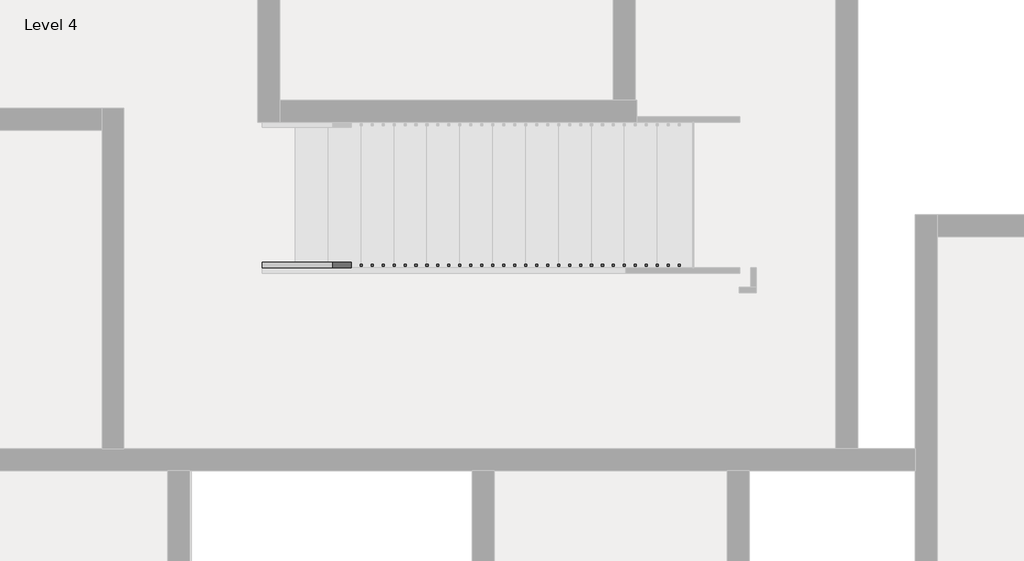
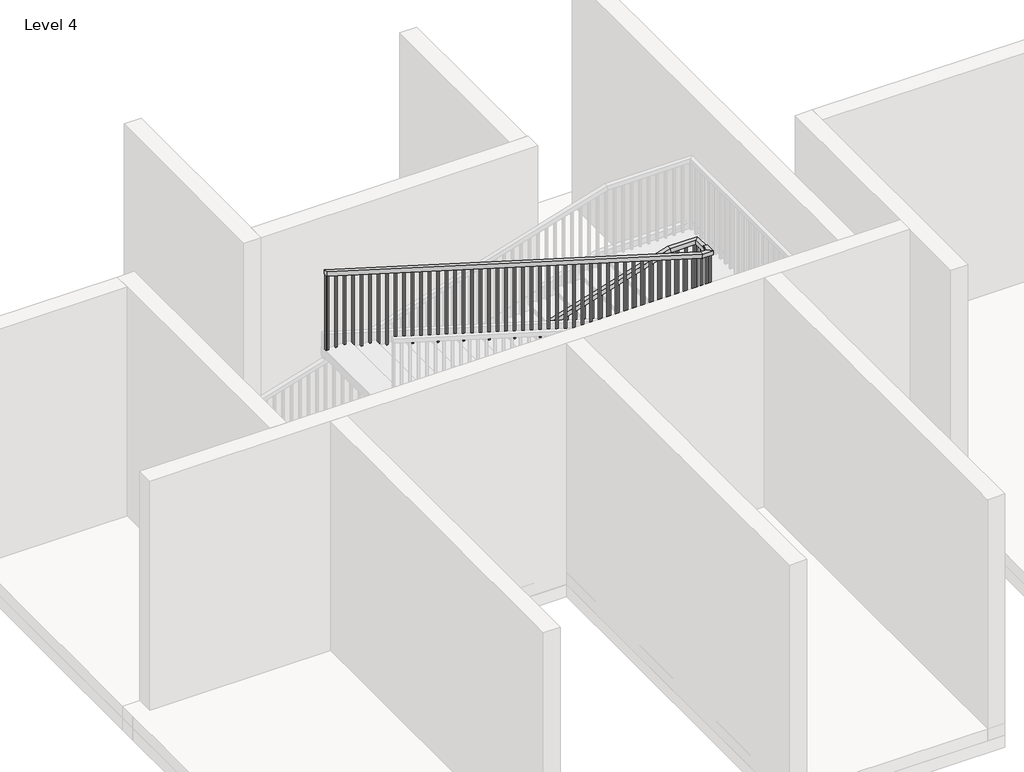
# One storey, part 11 of 14: 1 railing.
"""IFC4 building model written with IfcOpenShell, lengths in millimetres."""

from ifc_helpers import new_model, si_unit, frame, origin, place, context, project, spatial, polyline, outline, extrude, faceted_brep, element, save

model = new_model("IFC4")

# Units and contexts
model_context = context("Model", 3, world=origin())
ifc_project = project(units=[si_unit("LENGTHUNIT", "METRE", prefix="MILLI")], contexts=[model_context])

# Site, building, storey
site = spatial("IfcSite", under=ifc_project)
building = spatial("IfcBuilding", under=site)
storey = spatial("IfcBuildingStorey", under=building, Name="Level 4", Elevation=9144.0)

# Railing
placement = place(None, origin())
element("IfcRailing", 1, ObjectType="Handrail - Rectangular", at=placement, inside=storey, context=model_context, shape_type="SolidModel", body=[
    faceted_brep([(-5254.0891351, 11205.0082924, 10149.84), (-5254.0891351, 11205.0082924, 10096.8032429), (-5254.0891351, 11154.2082924, 10096.8032429), (-5254.0891351, 11154.2082924, 10149.84), (-986.8891351, 11205.0082924, 11430.0), (-979.4332782, 11205.0082924, 11379.2), (-979.4332782, 11154.2082924, 11379.2), (-986.8891351, 11154.2082924, 11430.0), (-631.2891351, 11205.0082924, 11430.0), (-631.2891351, 11205.0082924, 11379.2), (-682.0891351, 11154.2082924, 11379.2), (-682.0891351, 11154.2082924, 11430.0), (-631.2891351, 11001.8082924, 11430.0), (-631.2891351, 10951.0082924, 11379.2), (-682.0891351, 10951.0082924, 11379.2), (-682.0891351, 11001.8082924, 11430.0), (-631.2891351, 11001.8082924, 11452.86), (-631.2891351, 10951.0082924, 11402.06), (-682.0891351, 10951.0082924, 11402.06), (-682.0891351, 11001.8082924, 11452.86), (-631.2891351, 10874.8082924, 11452.86), (-631.2891351, 10874.8082924, 11402.06), (-682.0891351, 10925.6082924, 11402.06), (-682.0891351, 10925.6082924, 11452.86), (-758.2891351, 10874.8082924, 11452.86), (-765.744992, 10874.8082924, 11402.06), (-765.744992, 10925.6082924, 11402.06), (-758.2891351, 10925.6082924, 11452.86), (-5254.0891351, 10874.8082924, 12801.6), (-5254.0891351, 10925.6082924, 12801.6), (-5254.0891351, 10925.6082924, 12748.5632429), (-5254.0891351, 10874.8082924, 12748.5632429)], [[[0, 1, 2, 3]], [[1, 0, 4, 5]], [[2, 1, 5, 6]], [[3, 2, 6, 7]], [[0, 3, 7, 4]], [[5, 4, 8, 9]], [[6, 5, 9, 10]], [[7, 6, 10, 11]], [[4, 7, 11, 8]], [[9, 8, 12, 13]], [[10, 9, 13, 14]], [[11, 10, 14, 15]], [[8, 11, 15, 12]], [[13, 12, 16, 17]], [[14, 13, 17, 18]], [[15, 14, 18, 19]], [[12, 15, 19, 16]], [[17, 16, 20, 21]], [[18, 17, 21, 22]], [[19, 18, 22, 23]], [[16, 19, 23, 20]], [[21, 20, 24, 25]], [[22, 21, 25, 26]], [[23, 22, 26, 27]], [[20, 23, 27, 24]], [[28, 29, 30, 31]], [[25, 24, 28, 31]], [[26, 25, 31, 30]], [[27, 26, 30, 29]], [[24, 27, 29, 28]]]),
    extrude(outline(polyline([(12738.0857429, -5219.1641351), (12743.8007429, -5238.2141351), (11795.76, -5238.2141351), (11795.76, -5219.1641351), (12738.0857429, -5219.1641351)])), frame((0.0, 10890.6832924, 0.0), z_axis=(0.0, 1.0, 0.0), x_axis=(0.0, 0.0, 1.0)), (0.0, 0.0, 1.0), 19.05),
    extrude(outline(polyline([(12707.6057429, -5117.5641351), (12713.3207429, -5136.6141351), (11795.76, -5136.6141351), (11795.76, -5117.5641351), (12707.6057429, -5117.5641351)])), frame((0.0, 10890.6832924, 0.0), z_axis=(0.0, 1.0, 0.0), x_axis=(0.0, 0.0, 1.0)), (0.0, 0.0, 1.0), 19.05),
    extrude(outline(polyline([(12677.1257429, -5015.9641351), (12682.8407429, -5035.0141351), (11795.76, -5035.0141351), (11795.76, -5015.9641351), (12677.1257429, -5015.9641351)])), frame((0.0, 10890.6832924, 0.0), z_axis=(0.0, 1.0, 0.0), x_axis=(0.0, 0.0, 1.0)), (0.0, 0.0, 1.0), 19.05),
    extrude(outline(polyline([(12646.6457429, -4914.3641351), (12652.3607429, -4933.4141351), (11704.32, -4933.4141351), (11704.32, -4914.3641351), (12646.6457429, -4914.3641351)])), frame((0.0, 10890.6832924, 0.0), z_axis=(0.0, 1.0, 0.0), x_axis=(0.0, 0.0, 1.0)), (0.0, 0.0, 1.0), 19.05),
    extrude(outline(polyline([(12616.1657429, -4812.7641351), (12621.8807429, -4831.8141351), (11704.32, -4831.8141351), (11704.32, -4812.7641351), (12616.1657429, -4812.7641351)])), frame((0.0, 10890.6832924, 0.0), z_axis=(0.0, 1.0, 0.0), x_axis=(0.0, 0.0, 1.0)), (0.0, 0.0, 1.0), 19.05),
    extrude(outline(polyline([(12585.6857429, -4711.1641351), (12591.4007429, -4730.2141351), (11704.32, -4730.2141351), (11704.32, -4711.1641351), (12585.6857429, -4711.1641351)])), frame((0.0, 10890.6832924, 0.0), z_axis=(0.0, 1.0, 0.0), x_axis=(0.0, 0.0, 1.0)), (0.0, 0.0, 1.0), 19.05),
    extrude(outline(polyline([(12555.2057429, -4609.5641351), (12560.9207429, -4628.6141351), (11612.88, -4628.6141351), (11612.88, -4609.5641351), (12555.2057429, -4609.5641351)])), frame((0.0, 10890.6832924, 0.0), z_axis=(0.0, 1.0, 0.0), x_axis=(0.0, 0.0, 1.0)), (0.0, 0.0, 1.0), 19.05),
    extrude(outline(polyline([(12524.7257429, -4507.9641351), (12530.4407429, -4527.0141351), (11612.88, -4527.0141351), (11612.88, -4507.9641351), (12524.7257429, -4507.9641351)])), frame((0.0, 10890.6832924, 0.0), z_axis=(0.0, 1.0, 0.0), x_axis=(0.0, 0.0, 1.0)), (0.0, 0.0, 1.0), 19.05),
    extrude(outline(polyline([(12494.2457429, -4406.3641351), (12499.9607429, -4425.4141351), (11612.88, -4425.4141351), (11612.88, -4406.3641351), (12494.2457429, -4406.3641351)])), frame((0.0, 10890.6832924, 0.0), z_axis=(0.0, 1.0, 0.0), x_axis=(0.0, 0.0, 1.0)), (0.0, 0.0, 1.0), 19.05),
    extrude(outline(polyline([(12463.7657429, -4304.7641351), (12469.4807429, -4323.8141351), (11521.44, -4323.8141351), (11521.44, -4304.7641351), (12463.7657429, -4304.7641351)])), frame((0.0, 10890.6832924, 0.0), z_axis=(0.0, 1.0, 0.0), x_axis=(0.0, 0.0, 1.0)), (0.0, 0.0, 1.0), 19.05),
    extrude(outline(polyline([(12433.2857429, -4203.1641351), (12439.0007429, -4222.2141351), (11521.44, -4222.2141351), (11521.44, -4203.1641351), (12433.2857429, -4203.1641351)])), frame((0.0, 10890.6832924, 0.0), z_axis=(0.0, 1.0, 0.0), x_axis=(0.0, 0.0, 1.0)), (0.0, 0.0, 1.0), 19.05),
    extrude(outline(polyline([(12402.8057429, -4101.5641351), (12408.5207429, -4120.6141351), (11521.44, -4120.6141351), (11521.44, -4101.5641351), (12402.8057429, -4101.5641351)])), frame((0.0, 10890.6832924, 0.0), z_axis=(0.0, 1.0, 0.0), x_axis=(0.0, 0.0, 1.0)), (0.0, 0.0, 1.0), 19.05),
    extrude(outline(polyline([(12372.3257429, -3999.9641351), (12378.0407429, -4019.0141351), (11430.0, -4019.0141351), (11430.0, -3999.9641351), (12372.3257429, -3999.9641351)])), frame((0.0, 10890.6832924, 0.0), z_axis=(0.0, 1.0, 0.0), x_axis=(0.0, 0.0, 1.0)), (0.0, 0.0, 1.0), 19.05),
    extrude(outline(polyline([(12341.8457429, -3898.3641351), (12347.5607429, -3917.4141351), (11430.0, -3917.4141351), (11430.0, -3898.3641351), (12341.8457429, -3898.3641351)])), frame((0.0, 10890.6832924, 0.0), z_axis=(0.0, 1.0, 0.0), x_axis=(0.0, 0.0, 1.0)), (0.0, 0.0, 1.0), 19.05),
    extrude(outline(polyline([(12311.3657429, -3796.7641351), (12317.0807429, -3815.8141351), (11430.0, -3815.8141351), (11430.0, -3796.7641351), (12311.3657429, -3796.7641351)])), frame((0.0, 10890.6832924, 0.0), z_axis=(0.0, 1.0, 0.0), x_axis=(0.0, 0.0, 1.0)), (0.0, 0.0, 1.0), 19.05),
    extrude(outline(polyline([(12280.8857429, -3695.1641351), (12286.6007429, -3714.2141351), (11338.56, -3714.2141351), (11338.56, -3695.1641351), (12280.8857429, -3695.1641351)])), frame((0.0, 10890.6832924, 0.0), z_axis=(0.0, 1.0, 0.0), x_axis=(0.0, 0.0, 1.0)), (0.0, 0.0, 1.0), 19.05),
    extrude(outline(polyline([(12250.4057429, -3593.5641351), (12256.1207429, -3612.6141351), (11338.56, -3612.6141351), (11338.56, -3593.5641351), (12250.4057429, -3593.5641351)])), frame((0.0, 10890.6832924, 0.0), z_axis=(0.0, 1.0, 0.0), x_axis=(0.0, 0.0, 1.0)), (0.0, 0.0, 1.0), 19.05),
    extrude(outline(polyline([(12219.9257429, -3491.9641351), (12225.6407429, -3511.0141351), (11338.56, -3511.0141351), (11338.56, -3491.9641351), (12219.9257429, -3491.9641351)])), frame((0.0, 10890.6832924, 0.0), z_axis=(0.0, 1.0, 0.0), x_axis=(0.0, 0.0, 1.0)), (0.0, 0.0, 1.0), 19.05),
    extrude(outline(polyline([(12189.4457429, -3390.3641351), (12195.1607429, -3409.4141351), (11247.12, -3409.4141351), (11247.12, -3390.3641351), (12189.4457429, -3390.3641351)])), frame((0.0, 10890.6832924, 0.0), z_axis=(0.0, 1.0, 0.0), x_axis=(0.0, 0.0, 1.0)), (0.0, 0.0, 1.0), 19.05),
    extrude(outline(polyline([(12158.9657429, -3288.7641351), (12164.6807429, -3307.8141351), (11247.12, -3307.8141351), (11247.12, -3288.7641351), (12158.9657429, -3288.7641351)])), frame((0.0, 10890.6832924, 0.0), z_axis=(0.0, 1.0, 0.0), x_axis=(0.0, 0.0, 1.0)), (0.0, 0.0, 1.0), 19.05),
    extrude(outline(polyline([(12128.4857429, -3187.1641351), (12134.2007429, -3206.2141351), (11247.12, -3206.2141351), (11247.12, -3187.1641351), (12128.4857429, -3187.1641351)])), frame((0.0, 10890.6832924, 0.0), z_axis=(0.0, 1.0, 0.0), x_axis=(0.0, 0.0, 1.0)), (0.0, 0.0, 1.0), 19.05),
    extrude(outline(polyline([(12098.0057429, -3085.5641351), (12103.7207429, -3104.6141351), (11155.68, -3104.6141351), (11155.68, -3085.5641351), (12098.0057429, -3085.5641351)])), frame((0.0, 10890.6832924, 0.0), z_axis=(0.0, 1.0, 0.0), x_axis=(0.0, 0.0, 1.0)), (0.0, 0.0, 1.0), 19.05),
    extrude(outline(polyline([(12067.5257429, -2983.9641351), (12073.2407429, -3003.0141351), (11155.68, -3003.0141351), (11155.68, -2983.9641351), (12067.5257429, -2983.9641351)])), frame((0.0, 10890.6832924, 0.0), z_axis=(0.0, 1.0, 0.0), x_axis=(0.0, 0.0, 1.0)), (0.0, 0.0, 1.0), 19.05),
    extrude(outline(polyline([(12037.0457429, -2882.3641351), (12042.7607429, -2901.4141351), (11155.68, -2901.4141351), (11155.68, -2882.3641351), (12037.0457429, -2882.3641351)])), frame((0.0, 10890.6832924, 0.0), z_axis=(0.0, 1.0, 0.0), x_axis=(0.0, 0.0, 1.0)), (0.0, 0.0, 1.0), 19.05),
    extrude(outline(polyline([(12006.5657429, -2780.7641351), (12012.2807429, -2799.8141351), (11064.24, -2799.8141351), (11064.24, -2780.7641351), (12006.5657429, -2780.7641351)])), frame((0.0, 10890.6832924, 0.0), z_axis=(0.0, 1.0, 0.0), x_axis=(0.0, 0.0, 1.0)), (0.0, 0.0, 1.0), 19.05),
    extrude(outline(polyline([(11976.0857429, -2679.1641351), (11981.8007429, -2698.2141351), (11064.24, -2698.2141351), (11064.24, -2679.1641351), (11976.0857429, -2679.1641351)])), frame((0.0, 10890.6832924, 0.0), z_axis=(0.0, 1.0, 0.0), x_axis=(0.0, 0.0, 1.0)), (0.0, 0.0, 1.0), 19.05),
    extrude(outline(polyline([(11945.6057429, -2577.5641351), (11951.3207429, -2596.6141351), (11064.24, -2596.6141351), (11064.24, -2577.5641351), (11945.6057429, -2577.5641351)])), frame((0.0, 10890.6832924, 0.0), z_axis=(0.0, 1.0, 0.0), x_axis=(0.0, 0.0, 1.0)), (0.0, 0.0, 1.0), 19.05),
    extrude(outline(polyline([(11915.1257429, -2475.9641351), (11920.8407429, -2495.0141351), (10972.8, -2495.0141351), (10972.8, -2475.9641351), (11915.1257429, -2475.9641351)])), frame((0.0, 10890.6832924, 0.0), z_axis=(0.0, 1.0, 0.0), x_axis=(0.0, 0.0, 1.0)), (0.0, 0.0, 1.0), 19.05),
    extrude(outline(polyline([(11884.6457429, -2374.3641351), (11890.3607429, -2393.4141351), (10972.8, -2393.4141351), (10972.8, -2374.3641351), (11884.6457429, -2374.3641351)])), frame((0.0, 10890.6832924, 0.0), z_axis=(0.0, 1.0, 0.0), x_axis=(0.0, 0.0, 1.0)), (0.0, 0.0, 1.0), 19.05),
    extrude(outline(polyline([(11854.1657429, -2272.7641351), (11859.8807429, -2291.8141351), (10972.8, -2291.8141351), (10972.8, -2272.7641351), (11854.1657429, -2272.7641351)])), frame((0.0, 10890.6832924, 0.0), z_axis=(0.0, 1.0, 0.0), x_axis=(0.0, 0.0, 1.0)), (0.0, 0.0, 1.0), 19.05),
    extrude(outline(polyline([(11823.6857429, -2171.1641351), (11829.4007429, -2190.2141351), (10881.36, -2190.2141351), (10881.36, -2171.1641351), (11823.6857429, -2171.1641351)])), frame((0.0, 10890.6832924, 0.0), z_axis=(0.0, 1.0, 0.0), x_axis=(0.0, 0.0, 1.0)), (0.0, 0.0, 1.0), 19.05),
    extrude(outline(polyline([(11793.2057429, -2069.5641351), (11798.9207429, -2088.6141351), (10881.36, -2088.6141351), (10881.36, -2069.5641351), (11793.2057429, -2069.5641351)])), frame((0.0, 10890.6832924, 0.0), z_axis=(0.0, 1.0, 0.0), x_axis=(0.0, 0.0, 1.0)), (0.0, 0.0, 1.0), 19.05),
    extrude(outline(polyline([(11762.7257429, -1967.9641351), (11768.4407429, -1987.0141351), (10881.36, -1987.0141351), (10881.36, -1967.9641351), (11762.7257429, -1967.9641351)])), frame((0.0, 10890.6832924, 0.0), z_axis=(0.0, 1.0, 0.0), x_axis=(0.0, 0.0, 1.0)), (0.0, 0.0, 1.0), 19.05),
    extrude(outline(polyline([(11732.2457429, -1866.3641351), (11737.9607429, -1885.4141351), (10789.92, -1885.4141351), (10789.92, -1866.3641351), (11732.2457429, -1866.3641351)])), frame((0.0, 10890.6832924, 0.0), z_axis=(0.0, 1.0, 0.0), x_axis=(0.0, 0.0, 1.0)), (0.0, 0.0, 1.0), 19.05),
    extrude(outline(polyline([(11701.7657429, -1764.7641351), (11707.4807429, -1783.8141351), (10789.92, -1783.8141351), (10789.92, -1764.7641351), (11701.7657429, -1764.7641351)])), frame((0.0, 10890.6832924, 0.0), z_axis=(0.0, 1.0, 0.0), x_axis=(0.0, 0.0, 1.0)), (0.0, 0.0, 1.0), 19.05),
    extrude(outline(polyline([(11671.2857429, -1663.1641351), (11677.0007429, -1682.2141351), (10789.92, -1682.2141351), (10789.92, -1663.1641351), (11671.2857429, -1663.1641351)])), frame((0.0, 10890.6832924, 0.0), z_axis=(0.0, 1.0, 0.0), x_axis=(0.0, 0.0, 1.0)), (0.0, 0.0, 1.0), 19.05),
    extrude(outline(polyline([(11640.8057429, -1561.5641351), (11646.5207429, -1580.6141351), (10698.48, -1580.6141351), (10698.48, -1561.5641351), (11640.8057429, -1561.5641351)])), frame((0.0, 10890.6832924, 0.0), z_axis=(0.0, 1.0, 0.0), x_axis=(0.0, 0.0, 1.0)), (0.0, 0.0, 1.0), 19.05),
    extrude(outline(polyline([(11610.3257429, -1459.9641351), (11616.0407429, -1479.0141351), (10698.48, -1479.0141351), (10698.48, -1459.9641351), (11610.3257429, -1459.9641351)])), frame((0.0, 10890.6832924, 0.0), z_axis=(0.0, 1.0, 0.0), x_axis=(0.0, 0.0, 1.0)), (0.0, 0.0, 1.0), 19.05),
    extrude(outline(polyline([(11579.8457429, -1358.3641351), (11585.5607429, -1377.4141351), (10698.48, -1377.4141351), (10698.48, -1358.3641351), (11579.8457429, -1358.3641351)])), frame((0.0, 10890.6832924, 0.0), z_axis=(0.0, 1.0, 0.0), x_axis=(0.0, 0.0, 1.0)), (0.0, 0.0, 1.0), 19.05),
    extrude(outline(polyline([(11549.3657429, -1256.7641351), (11555.0807429, -1275.8141351), (10607.04, -1275.8141351), (10607.04, -1256.7641351), (11549.3657429, -1256.7641351)])), frame((0.0, 10890.6832924, 0.0), z_axis=(0.0, 1.0, 0.0), x_axis=(0.0, 0.0, 1.0)), (0.0, 0.0, 1.0), 19.05),
    extrude(outline(polyline([(11518.8857429, -1155.1641351), (11524.6007429, -1174.2141351), (10607.04, -1174.2141351), (10607.04, -1155.1641351), (11518.8857429, -1155.1641351)])), frame((0.0, 10890.6832924, 0.0), z_axis=(0.0, 1.0, 0.0), x_axis=(0.0, 0.0, 1.0)), (0.0, 0.0, 1.0), 19.05),
    extrude(outline(polyline([(11488.4057429, -1053.5641351), (11494.1207429, -1072.6141351), (10607.04, -1072.6141351), (10607.04, -1053.5641351), (11488.4057429, -1053.5641351)])), frame((0.0, 10890.6832924, 0.0), z_axis=(0.0, 1.0, 0.0), x_axis=(0.0, 0.0, 1.0)), (0.0, 0.0, 1.0), 19.05),
    extrude(outline(polyline([(11457.9257429, -951.9641351), (11463.6407429, -971.0141351), (10515.6, -971.0141351), (10515.6, -951.9641351), (11457.9257429, -951.9641351)])), frame((0.0, 10890.6832924, 0.0), z_axis=(0.0, 1.0, 0.0), x_axis=(0.0, 0.0, 1.0)), (0.0, 0.0, 1.0), 19.05),
    extrude(outline(polyline([(11427.4457429, -850.3641351), (11433.1607429, -869.4141351), (10515.6, -869.4141351), (10515.6, -850.3641351), (11427.4457429, -850.3641351)])), frame((0.0, 10890.6832924, 0.0), z_axis=(0.0, 1.0, 0.0), x_axis=(0.0, 0.0, 1.0)), (0.0, 0.0, 1.0), 19.05),
    extrude(outline(polyline([(11396.9657429, -748.7641351), (11402.6807429, -767.8141351), (10515.6, -767.8141351), (10515.6, -748.7641351), (11396.9657429, -748.7641351)])), frame((0.0, 10890.6832924, 0.0), z_axis=(0.0, 1.0, 0.0), x_axis=(0.0, 0.0, 1.0)), (0.0, 0.0, 1.0), 19.05),
    extrude(outline(polyline([(-666.2141351, 10985.9332924), (-647.1641351, 10985.9332924), (-647.1641351, 10966.8832924), (-666.2141351, 10966.8832924), (-666.2141351, 10985.9332924)])), frame((0.0, 0.0, 10515.6), z_axis=(0.0, 0.0, 1.0), x_axis=(1.0, 0.0, 0.0)), (0.0, 0.0, 1.0), 886.46),
    extrude(outline(polyline([(-666.2141351, 11087.5332924), (-647.1641351, 11087.5332924), (-647.1641351, 11068.4832924), (-666.2141351, 11068.4832924), (-666.2141351, 11087.5332924)])), frame((0.0, 0.0, 10515.6), z_axis=(0.0, 0.0, 1.0), x_axis=(1.0, 0.0, 0.0)), (0.0, 0.0, 1.0), 863.6),
    extrude(outline(polyline([(-691.6141351, 11170.0832924), (-691.6141351, 11189.1332924), (-672.5641351, 11189.1332924), (-672.5641351, 11170.0832924), (-691.6141351, 11170.0832924)])), frame((0.0, 0.0, 10515.6), z_axis=(0.0, 0.0, 1.0), x_axis=(1.0, 0.0, 0.0)), (0.0, 0.0, 1.0), 863.6),
    extrude(outline(polyline([(-793.2141351, 11170.0832924), (-793.2141351, 11189.1332924), (-774.1641351, 11189.1332924), (-774.1641351, 11170.0832924), (-793.2141351, 11170.0832924)])), frame((0.0, 0.0, 10515.6), z_axis=(0.0, 0.0, 1.0), x_axis=(1.0, 0.0, 0.0)), (0.0, 0.0, 1.0), 863.6),
    extrude(outline(polyline([(-894.8141351, 11170.0832924), (-894.8141351, 11189.1332924), (-875.7641351, 11189.1332924), (-875.7641351, 11170.0832924), (-894.8141351, 11170.0832924)])), frame((0.0, 0.0, 10515.6), z_axis=(0.0, 0.0, 1.0), x_axis=(1.0, 0.0, 0.0)), (0.0, 0.0, 1.0), 863.6),
    extrude(outline(polyline([(11379.8207429, -977.3641351), (11374.1057429, -996.4141351), (10515.6, -996.4141351), (10515.6, -977.3641351), (11379.8207429, -977.3641351)])), frame((0.0, 11170.0832924, 0.0), z_axis=(0.0, 1.0, 0.0), x_axis=(0.0, 0.0, 1.0)), (0.0, 0.0, 1.0), 19.05),
    extrude(outline(polyline([(11349.3407429, -1078.9641351), (11343.6257429, -1098.0141351), (10424.16, -1098.0141351), (10424.16, -1078.9641351), (11349.3407429, -1078.9641351)])), frame((0.0, 11170.0832924, 0.0), z_axis=(0.0, 1.0, 0.0), x_axis=(0.0, 0.0, 1.0)), (0.0, 0.0, 1.0), 19.05),
    extrude(outline(polyline([(11318.8607429, -1180.5641351), (11313.1457429, -1199.6141351), (10424.16, -1199.6141351), (10424.16, -1180.5641351), (11318.8607429, -1180.5641351)])), frame((0.0, 11170.0832924, 0.0), z_axis=(0.0, 1.0, 0.0), x_axis=(0.0, 0.0, 1.0)), (0.0, 0.0, 1.0), 19.05),
    extrude(outline(polyline([(11288.3807429, -1282.1641351), (11282.6657429, -1301.2141351), (10424.16, -1301.2141351), (10424.16, -1282.1641351), (11288.3807429, -1282.1641351)])), frame((0.0, 11170.0832924, 0.0), z_axis=(0.0, 1.0, 0.0), x_axis=(0.0, 0.0, 1.0)), (0.0, 0.0, 1.0), 19.05),
    extrude(outline(polyline([(11257.9007429, -1383.7641351), (11252.1857429, -1402.8141351), (10332.72, -1402.8141351), (10332.72, -1383.7641351), (11257.9007429, -1383.7641351)])), frame((0.0, 11170.0832924, 0.0), z_axis=(0.0, 1.0, 0.0), x_axis=(0.0, 0.0, 1.0)), (0.0, 0.0, 1.0), 19.05),
    extrude(outline(polyline([(11227.4207429, -1485.3641351), (11221.7057429, -1504.4141351), (10332.72, -1504.4141351), (10332.72, -1485.3641351), (11227.4207429, -1485.3641351)])), frame((0.0, 11170.0832924, 0.0), z_axis=(0.0, 1.0, 0.0), x_axis=(0.0, 0.0, 1.0)), (0.0, 0.0, 1.0), 19.05),
    extrude(outline(polyline([(11196.9407429, -1586.9641351), (11191.2257429, -1606.0141351), (10332.72, -1606.0141351), (10332.72, -1586.9641351), (11196.9407429, -1586.9641351)])), frame((0.0, 11170.0832924, 0.0), z_axis=(0.0, 1.0, 0.0), x_axis=(0.0, 0.0, 1.0)), (0.0, 0.0, 1.0), 19.05),
    extrude(outline(polyline([(11166.4607429, -1688.5641351), (11160.7457429, -1707.6141351), (10241.28, -1707.6141351), (10241.28, -1688.5641351), (11166.4607429, -1688.5641351)])), frame((0.0, 11170.0832924, 0.0), z_axis=(0.0, 1.0, 0.0), x_axis=(0.0, 0.0, 1.0)), (0.0, 0.0, 1.0), 19.05),
    extrude(outline(polyline([(11135.9807429, -1790.1641351), (11130.2657429, -1809.2141351), (10241.28, -1809.2141351), (10241.28, -1790.1641351), (11135.9807429, -1790.1641351)])), frame((0.0, 11170.0832924, 0.0), z_axis=(0.0, 1.0, 0.0), x_axis=(0.0, 0.0, 1.0)), (0.0, 0.0, 1.0), 19.05),
    extrude(outline(polyline([(11105.5007429, -1891.7641351), (11099.7857429, -1910.8141351), (10241.28, -1910.8141351), (10241.28, -1891.7641351), (11105.5007429, -1891.7641351)])), frame((0.0, 11170.0832924, 0.0), z_axis=(0.0, 1.0, 0.0), x_axis=(0.0, 0.0, 1.0)), (0.0, 0.0, 1.0), 19.05),
    extrude(outline(polyline([(11075.0207429, -1993.3641351), (11069.3057429, -2012.4141351), (10149.84, -2012.4141351), (10149.84, -1993.3641351), (11075.0207429, -1993.3641351)])), frame((0.0, 11170.0832924, 0.0), z_axis=(0.0, 1.0, 0.0), x_axis=(0.0, 0.0, 1.0)), (0.0, 0.0, 1.0), 19.05),
    extrude(outline(polyline([(11044.5407429, -2094.9641351), (11038.8257429, -2114.0141351), (10149.84, -2114.0141351), (10149.84, -2094.9641351), (11044.5407429, -2094.9641351)])), frame((0.0, 11170.0832924, 0.0), z_axis=(0.0, 1.0, 0.0), x_axis=(0.0, 0.0, 1.0)), (0.0, 0.0, 1.0), 19.05),
    extrude(outline(polyline([(11014.0607429, -2196.5641351), (11008.3457429, -2215.6141351), (10149.84, -2215.6141351), (10149.84, -2196.5641351), (11014.0607429, -2196.5641351)])), frame((0.0, 11170.0832924, 0.0), z_axis=(0.0, 1.0, 0.0), x_axis=(0.0, 0.0, 1.0)), (0.0, 0.0, 1.0), 19.05),
    extrude(outline(polyline([(10983.5807429, -2298.1641351), (10977.8657429, -2317.2141351), (10058.4, -2317.2141351), (10058.4, -2298.1641351), (10983.5807429, -2298.1641351)])), frame((0.0, 11170.0832924, 0.0), z_axis=(0.0, 1.0, 0.0), x_axis=(0.0, 0.0, 1.0)), (0.0, 0.0, 1.0), 19.05),
    extrude(outline(polyline([(10953.1007429, -2399.7641351), (10947.3857429, -2418.8141351), (10058.4, -2418.8141351), (10058.4, -2399.7641351), (10953.1007429, -2399.7641351)])), frame((0.0, 11170.0832924, 0.0), z_axis=(0.0, 1.0, 0.0), x_axis=(0.0, 0.0, 1.0)), (0.0, 0.0, 1.0), 19.05),
    extrude(outline(polyline([(10922.6207429, -2501.3641351), (10916.9057429, -2520.4141351), (10058.4, -2520.4141351), (10058.4, -2501.3641351), (10922.6207429, -2501.3641351)])), frame((0.0, 11170.0832924, 0.0), z_axis=(0.0, 1.0, 0.0), x_axis=(0.0, 0.0, 1.0)), (0.0, 0.0, 1.0), 19.05),
    extrude(outline(polyline([(10892.1407429, -2602.9641351), (10886.4257429, -2622.0141351), (9966.96, -2622.0141351), (9966.96, -2602.9641351), (10892.1407429, -2602.9641351)])), frame((0.0, 11170.0832924, 0.0), z_axis=(0.0, 1.0, 0.0), x_axis=(0.0, 0.0, 1.0)), (0.0, 0.0, 1.0), 19.05),
    extrude(outline(polyline([(10861.6607429, -2704.5641351), (10855.9457429, -2723.6141351), (9966.96, -2723.6141351), (9966.96, -2704.5641351), (10861.6607429, -2704.5641351)])), frame((0.0, 11170.0832924, 0.0), z_axis=(0.0, 1.0, 0.0), x_axis=(0.0, 0.0, 1.0)), (0.0, 0.0, 1.0), 19.05),
    extrude(outline(polyline([(10831.1807429, -2806.1641351), (10825.4657429, -2825.2141351), (9966.96, -2825.2141351), (9966.96, -2806.1641351), (10831.1807429, -2806.1641351)])), frame((0.0, 11170.0832924, 0.0), z_axis=(0.0, 1.0, 0.0), x_axis=(0.0, 0.0, 1.0)), (0.0, 0.0, 1.0), 19.05),
    extrude(outline(polyline([(10800.7007429, -2907.7641351), (10794.9857429, -2926.8141351), (9875.52, -2926.8141351), (9875.52, -2907.7641351), (10800.7007429, -2907.7641351)])), frame((0.0, 11170.0832924, 0.0), z_axis=(0.0, 1.0, 0.0), x_axis=(0.0, 0.0, 1.0)), (0.0, 0.0, 1.0), 19.05),
    extrude(outline(polyline([(10770.2207429, -3009.3641351), (10764.5057429, -3028.4141351), (9875.52, -3028.4141351), (9875.52, -3009.3641351), (10770.2207429, -3009.3641351)])), frame((0.0, 11170.0832924, 0.0), z_axis=(0.0, 1.0, 0.0), x_axis=(0.0, 0.0, 1.0)), (0.0, 0.0, 1.0), 19.05),
    extrude(outline(polyline([(10739.7407429, -3110.9641351), (10734.0257429, -3130.0141351), (9875.52, -3130.0141351), (9875.52, -3110.9641351), (10739.7407429, -3110.9641351)])), frame((0.0, 11170.0832924, 0.0), z_axis=(0.0, 1.0, 0.0), x_axis=(0.0, 0.0, 1.0)), (0.0, 0.0, 1.0), 19.05),
    extrude(outline(polyline([(10709.2607429, -3212.5641351), (10703.5457429, -3231.6141351), (9784.08, -3231.6141351), (9784.08, -3212.5641351), (10709.2607429, -3212.5641351)])), frame((0.0, 11170.0832924, 0.0), z_axis=(0.0, 1.0, 0.0), x_axis=(0.0, 0.0, 1.0)), (0.0, 0.0, 1.0), 19.05),
    extrude(outline(polyline([(10678.7807429, -3314.1641351), (10673.0657429, -3333.2141351), (9784.08, -3333.2141351), (9784.08, -3314.1641351), (10678.7807429, -3314.1641351)])), frame((0.0, 11170.0832924, 0.0), z_axis=(0.0, 1.0, 0.0), x_axis=(0.0, 0.0, 1.0)), (0.0, 0.0, 1.0), 19.05),
    extrude(outline(polyline([(10648.3007429, -3415.7641351), (10642.5857429, -3434.8141351), (9784.08, -3434.8141351), (9784.08, -3415.7641351), (10648.3007429, -3415.7641351)])), frame((0.0, 11170.0832924, 0.0), z_axis=(0.0, 1.0, 0.0), x_axis=(0.0, 0.0, 1.0)), (0.0, 0.0, 1.0), 19.05),
    extrude(outline(polyline([(10617.8207429, -3517.3641351), (10612.1057429, -3536.4141351), (9692.64, -3536.4141351), (9692.64, -3517.3641351), (10617.8207429, -3517.3641351)])), frame((0.0, 11170.0832924, 0.0), z_axis=(0.0, 1.0, 0.0), x_axis=(0.0, 0.0, 1.0)), (0.0, 0.0, 1.0), 19.05),
    extrude(outline(polyline([(10587.3407429, -3618.9641351), (10581.6257429, -3638.0141351), (9692.64, -3638.0141351), (9692.64, -3618.9641351), (10587.3407429, -3618.9641351)])), frame((0.0, 11170.0832924, 0.0), z_axis=(0.0, 1.0, 0.0), x_axis=(0.0, 0.0, 1.0)), (0.0, 0.0, 1.0), 19.05),
    extrude(outline(polyline([(10556.8607429, -3720.5641351), (10551.1457429, -3739.6141351), (9692.64, -3739.6141351), (9692.64, -3720.5641351), (10556.8607429, -3720.5641351)])), frame((0.0, 11170.0832924, 0.0), z_axis=(0.0, 1.0, 0.0), x_axis=(0.0, 0.0, 1.0)), (0.0, 0.0, 1.0), 19.05),
    extrude(outline(polyline([(10526.3807429, -3822.1641351), (10520.6657429, -3841.2141351), (9601.2, -3841.2141351), (9601.2, -3822.1641351), (10526.3807429, -3822.1641351)])), frame((0.0, 11170.0832924, 0.0), z_axis=(0.0, 1.0, 0.0), x_axis=(0.0, 0.0, 1.0)), (0.0, 0.0, 1.0), 19.05),
    extrude(outline(polyline([(10495.9007429, -3923.7641351), (10490.1857429, -3942.8141351), (9601.2, -3942.8141351), (9601.2, -3923.7641351), (10495.9007429, -3923.7641351)])), frame((0.0, 11170.0832924, 0.0), z_axis=(0.0, 1.0, 0.0), x_axis=(0.0, 0.0, 1.0)), (0.0, 0.0, 1.0), 19.05),
    extrude(outline(polyline([(10465.4207429, -4025.3641351), (10459.7057429, -4044.4141351), (9601.2, -4044.4141351), (9601.2, -4025.3641351), (10465.4207429, -4025.3641351)])), frame((0.0, 11170.0832924, 0.0), z_axis=(0.0, 1.0, 0.0), x_axis=(0.0, 0.0, 1.0)), (0.0, 0.0, 1.0), 19.05),
    extrude(outline(polyline([(10434.9407429, -4126.9641351), (10429.2257429, -4146.0141351), (9509.76, -4146.0141351), (9509.76, -4126.9641351), (10434.9407429, -4126.9641351)])), frame((0.0, 11170.0832924, 0.0), z_axis=(0.0, 1.0, 0.0), x_axis=(0.0, 0.0, 1.0)), (0.0, 0.0, 1.0), 19.05),
    extrude(outline(polyline([(10404.4607429, -4228.5641351), (10398.7457429, -4247.6141351), (9509.76, -4247.6141351), (9509.76, -4228.5641351), (10404.4607429, -4228.5641351)])), frame((0.0, 11170.0832924, 0.0), z_axis=(0.0, 1.0, 0.0), x_axis=(0.0, 0.0, 1.0)), (0.0, 0.0, 1.0), 19.05),
    extrude(outline(polyline([(10373.9807429, -4330.1641351), (10368.2657429, -4349.2141351), (9509.76, -4349.2141351), (9509.76, -4330.1641351), (10373.9807429, -4330.1641351)])), frame((0.0, 11170.0832924, 0.0), z_axis=(0.0, 1.0, 0.0), x_axis=(0.0, 0.0, 1.0)), (0.0, 0.0, 1.0), 19.05),
    extrude(outline(polyline([(10343.5007429, -4431.7641351), (10337.7857429, -4450.8141351), (9418.32, -4450.8141351), (9418.32, -4431.7641351), (10343.5007429, -4431.7641351)])), frame((0.0, 11170.0832924, 0.0), z_axis=(0.0, 1.0, 0.0), x_axis=(0.0, 0.0, 1.0)), (0.0, 0.0, 1.0), 19.05),
    extrude(outline(polyline([(10313.0207429, -4533.3641351), (10307.3057429, -4552.4141351), (9418.32, -4552.4141351), (9418.32, -4533.3641351), (10313.0207429, -4533.3641351)])), frame((0.0, 11170.0832924, 0.0), z_axis=(0.0, 1.0, 0.0), x_axis=(0.0, 0.0, 1.0)), (0.0, 0.0, 1.0), 19.05),
    extrude(outline(polyline([(10282.5407429, -4634.9641351), (10276.8257429, -4654.0141351), (9418.32, -4654.0141351), (9418.32, -4634.9641351), (10282.5407429, -4634.9641351)])), frame((0.0, 11170.0832924, 0.0), z_axis=(0.0, 1.0, 0.0), x_axis=(0.0, 0.0, 1.0)), (0.0, 0.0, 1.0), 19.05),
    extrude(outline(polyline([(10252.0607429, -4736.5641351), (10246.3457429, -4755.6141351), (9326.88, -4755.6141351), (9326.88, -4736.5641351), (10252.0607429, -4736.5641351)])), frame((0.0, 11170.0832924, 0.0), z_axis=(0.0, 1.0, 0.0), x_axis=(0.0, 0.0, 1.0)), (0.0, 0.0, 1.0), 19.05),
    extrude(outline(polyline([(10221.5807429, -4838.1641351), (10215.8657429, -4857.2141351), (9326.88, -4857.2141351), (9326.88, -4838.1641351), (10221.5807429, -4838.1641351)])), frame((0.0, 11170.0832924, 0.0), z_axis=(0.0, 1.0, 0.0), x_axis=(0.0, 0.0, 1.0)), (0.0, 0.0, 1.0), 19.05),
    extrude(outline(polyline([(10191.1007429, -4939.7641351), (10185.3857429, -4958.8141351), (9326.88, -4958.8141351), (9326.88, -4939.7641351), (10191.1007429, -4939.7641351)])), frame((0.0, 11170.0832924, 0.0), z_axis=(0.0, 1.0, 0.0), x_axis=(0.0, 0.0, 1.0)), (0.0, 0.0, 1.0), 19.05),
    extrude(outline(polyline([(10160.6207429, -5041.3641351), (10154.9057429, -5060.4141351), (9235.44, -5060.4141351), (9235.44, -5041.3641351), (10160.6207429, -5041.3641351)])), frame((0.0, 11170.0832924, 0.0), z_axis=(0.0, 1.0, 0.0), x_axis=(0.0, 0.0, 1.0)), (0.0, 0.0, 1.0), 19.05),
    extrude(outline(polyline([(10130.1407429, -5142.9641351), (10124.4257429, -5162.0141351), (9235.44, -5162.0141351), (9235.44, -5142.9641351), (10130.1407429, -5142.9641351)])), frame((0.0, 11170.0832924, 0.0), z_axis=(0.0, 1.0, 0.0), x_axis=(0.0, 0.0, 1.0)), (0.0, 0.0, 1.0), 19.05),
    extrude(outline(polyline([(-666.2141351, 10909.7332924), (-647.1641351, 10909.7332924), (-647.1641351, 10890.6832924), (-666.2141351, 10890.6832924), (-666.2141351, 10909.7332924)])), frame((0.0, 0.0, 10515.6), z_axis=(0.0, 0.0, 1.0), x_axis=(1.0, 0.0, 0.0)), (0.0, 0.0, 1.0), 886.46),
    extrude(outline(polyline([(-666.2141351, 11170.0832924), (-666.2141351, 11189.1332924), (-647.1641351, 11189.1332924), (-647.1641351, 11170.0832924), (-666.2141351, 11170.0832924)])), frame((0.0, 0.0, 10515.6), z_axis=(0.0, 0.0, 1.0), x_axis=(1.0, 0.0, 0.0)), (0.0, 0.0, 1.0), 863.6),
    extrude(outline(polyline([(12742.8482429, -5235.0391351), (12748.5632429, -5254.0891351), (11795.76, -5254.0891351), (11795.76, -5235.0391351), (12742.8482429, -5235.0391351)])), frame((0.0, 10890.6832924, 0.0), z_axis=(0.0, 1.0, 0.0), x_axis=(0.0, 0.0, 1.0)), (0.0, 0.0, 1.0), 19.05),
    extrude(outline(polyline([(10102.5182429, -5235.0391351), (10096.8032429, -5254.0891351), (9235.44, -5254.0891351), (9235.44, -5235.0391351), (10102.5182429, -5235.0391351)])), frame((0.0, 11170.0832924, 0.0), z_axis=(0.0, 1.0, 0.0), x_axis=(0.0, 0.0, 1.0)), (0.0, 0.0, 1.0), 19.05),
])

save(model, "model.ifc")

# Revit data of these elements
# Type "Handrail - Rectangular"
#   Assembly Code = "C2010400"
#   built-in parameter 1008612 = 0.0416667 (stored number, unit not read)
#   built-in parameter 1008611 = 0.0416667 (stored number, unit not read)
#   built-in parameter 1008609 = 0.333333 (stored number, unit not read)
#   built-in parameter 1008604 = 0.166667 (stored number, unit not read)
#   built-in parameter 1008603 = 0.166667 (stored number, unit not read)
#   Railing Height = 3' - 0"
#   built-in parameter 1008630 = 2
#   built-in parameter 1008610 = 2
#   built-in parameter 1008618 = Baluster - Square : 3/4"
# Element 1 (IfcRailing, "Handrail - Rectangular")
#   Phase Created = New Construction
